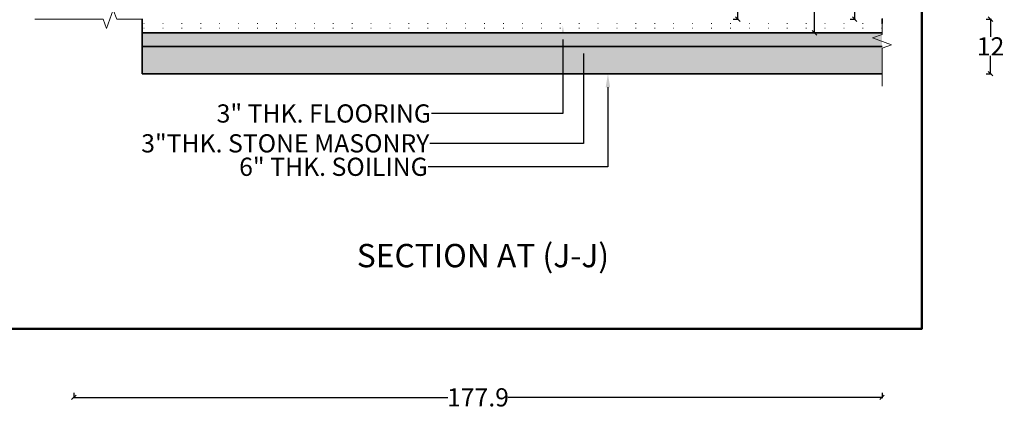
# Model space of a CAD drawing. Units: inches. Extents: x -60 to 284, y -245 to 257.
# Tile 2 of 10: x 55 to 272, y -245 to -159. Entities that reach past the tile are written whole.
import ezdxf
from ezdxf import colors
from ezdxf.entities.mleader import LeaderData, LeaderLine
from ezdxf.math import Vec2, Vec3

# ---------------------------------------------------------------- set-up
doc = ezdxf.new("R2010")
doc.units = ezdxf.units.IN
doc.header["$LTSCALE"] = 0.8
doc.header["$MEASUREMENT"] = 0
doc.linetypes.add('DOT', pattern=[6.35, 0, -6.35])
for name, color, linetype, lineweight in [('A-ANNO-DIMS', 2, 'Continuous', 18), ('A-ANNO-SYMB', 3, 'Continuous', 18), ('A-ANNO-TEXT', 3, 'Continuous', 18), ('A-ANNO-TTLB', 7, 'Continuous', 50), ('A-SECT', 7, 'Continuous', 35), ('A-SECT-OVHD', 8, 'DOT', 18), ('A-SECT-PATT', 8, 'Continuous', 13)]:
    doc.layers.add(name, color=color, linetype=linetype, lineweight=lineweight)
doc.styles.get("Standard").update_dxf_attribs({"font": 'arial.ttf'})
doc.dimstyles.get("Standard").update_dxf_attribs({"dimtxt": 4, "dimasz": 1, "dimexe": 0.18, "dimexo": 0.0625, "dimgap": 0.09, "dimtad": 0, "dimtih": 1, "dimtoh": 1, "dimzin": 0, "dimdsep": 46, "dimlunit": 4, "dimtxsty": 'Standard', "dimblk": 'OBLIQUE', "dimcen": 0.09, "dimadec": 0, "dimazin": 0, "dimtfac": 1, "dimtofl": 0, "dimtmove": 0, "dimatfit": 3, "dimfxl": 1, "dimfxlon": 1, "dimtolj": 1, "dimtzin": 0, "dimarcsym": 0})

# ---------------------------------------------------------------- blocks, each defined once
blk = doc.blocks.new('_Oblique')
at = {"color": 0, "linetype": 'ByBlock', "lineweight": -2}
blk.add_line((-0.5, -0.5), (0.5, 0.5), dxfattribs=at)
blk = doc.blocks.new('*D41')
at = {"layer": 'A-ANNO-DIMS', "color": 0, "lineweight": -2, "ltscale": 0.8, "transparency": 16777216}
for p, q in [((192.1, -91.86), (192.1, -90.68)), ((192.1, -90.86), (193.35, -90.86)), ((202.1, -90.86), (200.85, -90.86)), ((202.1, -91.86), (202.1, -90.68))]:
    blk.add_line(p, q, dxfattribs=at)
at = {"layer": 'Defpoints', "color": 0, "ltscale": 0.8, "transparency": 16777216}
for p in [(192.1, -90.86), (192.1, -168.75), (202.1, -168.75)]:
    blk.add_point(p, dxfattribs=at)
at = {"layer": 'A-ANNO-DIMS', "color": 0, "lineweight": -2, "ltscale": 0.8, "transparency": 16777216, "rotation": 180}
blk.add_blockref('_Oblique', (192.1, -90.86), dxfattribs=at)
at = {"layer": 'A-ANNO-DIMS', "color": 0, "lineweight": -2, "ltscale": 0.8, "transparency": 16777216}
blk.add_blockref('_Oblique', (202.1, -90.86), dxfattribs=at)
at = {"layer": 'A-ANNO-DIMS', "color": 0, "ltscale": 0.8, "transparency": 16777216, "insert": (197.1, -90.86), "char_height": 4, "attachment_point": 5}
blk.add_mtext('\\A1;10"', dxfattribs=at)
blk = doc.blocks.new('*D42')
at = {"layer": 'A-ANNO-DIMS', "color": 0, "lineweight": -2, "ltscale": 0.8, "transparency": 16777216}
for p, q in [((182.1, -91.86), (182.1, -90.68)), ((182.1, -90.86), (183.35, -90.86)), ((192.1, -90.86), (190.85, -90.86)), ((192.1, -91.86), (192.1, -90.68))]:
    blk.add_line(p, q, dxfattribs=at)
at = {"layer": 'Defpoints', "color": 0, "ltscale": 0.8, "transparency": 16777216}
for p in [(182.1, -90.86), (182.1, -162.75), (192.1, -162.75)]:
    blk.add_point(p, dxfattribs=at)
at = {"layer": 'A-ANNO-DIMS', "color": 0, "lineweight": -2, "ltscale": 0.8, "transparency": 16777216, "rotation": 180}
blk.add_blockref('_Oblique', (182.1, -90.86), dxfattribs=at)
at = {"layer": 'A-ANNO-DIMS', "color": 0, "lineweight": -2, "ltscale": 0.8, "transparency": 16777216}
blk.add_blockref('_Oblique', (192.1, -90.86), dxfattribs=at)
at = {"layer": 'A-ANNO-DIMS', "color": 0, "ltscale": 0.8, "transparency": 16777216, "insert": (187.1, -90.86), "char_height": 4, "attachment_point": 5}
blk.add_mtext('\\A1;10"', dxfattribs=at)
blk = doc.blocks.new('*D69')
at = {"layer": 'A-ANNO-DIMS', "color": 0, "lineweight": -2, "ltscale": 0.8, "transparency": 16777216}
for p, q in [((212.15, -46.21), (213.33, -46.21)), ((213.15, -46.21), (213.15, -100.58)), ((213.15, -159.21), (213.15, -104.84)), ((212.15, -159.21), (213.33, -159.21))]:
    blk.add_line(p, q, dxfattribs=at)
at = {"layer": 'Defpoints', "color": 0, "ltscale": 0.8, "transparency": 16777216}
for p in [(212.05, -46.21), (213.15, -46.21), (212.05, -159.21)]:
    blk.add_point(p, dxfattribs=at)
at = {"layer": 'A-ANNO-DIMS', "color": 0, "lineweight": -2, "ltscale": 0.8, "transparency": 16777216}
for p, rotation in [((213.15, -46.21), 90), ((213.15, -159.21), 270)]:
    blk.add_blockref('_Oblique', p, dxfattribs=dict(at, rotation=rotation))
at = {"layer": 'A-ANNO-DIMS', "color": 0, "ltscale": 0.8, "transparency": 16777216, "insert": (213.15, -102.71), "char_height": 4, "attachment_point": 5}
blk.add_mtext('\\A1;9\'-5"', dxfattribs=at)
blk = doc.blocks.new('*D70')
at = {"layer": 'A-ANNO-DIMS', "color": 0, "lineweight": -2, "ltscale": 0.8, "transparency": 16777216}
for p, q in [((229.03, -46.21), (230.21, -46.21)), ((230.03, -46.21), (230.03, -102.08)), ((230.03, -162.21), (230.03, -106.34)), ((229.03, -162.21), (230.21, -162.21))]:
    blk.add_line(p, q, dxfattribs=at)
at = {"layer": 'Defpoints', "color": 0, "ltscale": 0.8, "transparency": 16777216}
for p in [(227.81, -46.21), (230.03, -46.21), (219.24, -162.21)]:
    blk.add_point(p, dxfattribs=at)
at = {"layer": 'A-ANNO-DIMS', "color": 0, "lineweight": -2, "ltscale": 0.8, "transparency": 16777216}
for p, rotation in [((230.03, -46.21), 90), ((230.03, -162.21), 270)]:
    blk.add_blockref('_Oblique', p, dxfattribs=dict(at, rotation=rotation))
at = {"layer": 'A-ANNO-DIMS', "color": 0, "ltscale": 0.8, "transparency": 16777216, "insert": (230.03, -104.21), "char_height": 4, "attachment_point": 5}
blk.add_mtext('\\A1;9\'-8"', dxfattribs=at)
blk = doc.blocks.new('*D71')
at = {"layer": 'A-ANNO-DIMS', "color": 0, "lineweight": -2, "ltscale": 0.8, "transparency": 16777216}
for p, q in [((237.88, -38.61), (239.06, -38.61)), ((238.88, -38.61), (238.88, -94.1)), ((238.88, -159.21), (238.88, -103.72)), ((237.88, -159.21), (239.06, -159.21))]:
    blk.add_line(p, q, dxfattribs=at)
at = {"layer": 'Defpoints', "color": 0, "ltscale": 0.8, "transparency": 16777216}
for p in [(235.46, -38.61), (238.88, -38.61), (235.46, -159.21)]:
    blk.add_point(p, dxfattribs=at)
at = {"layer": 'A-ANNO-DIMS', "color": 0, "lineweight": -2, "ltscale": 0.8, "transparency": 16777216}
for p, rotation in [((238.88, -38.61), 90), ((238.88, -159.21), 270)]:
    blk.add_blockref('_Oblique', p, dxfattribs=dict(at, rotation=rotation))
at = {"layer": 'A-ANNO-DIMS', "color": 0, "ltscale": 0.8, "transparency": 16777216, "insert": (238.88, -98.91), "char_height": 4, "attachment_point": 5}
blk.add_mtext('\\A1;10\'-0{\\H1x;\\S1/2;}"', dxfattribs=at)
blk = doc.blocks.new('*D105')
at = {"layer": 'A-ANNO-DIMS', "color": 0, "lineweight": -2, "ltscale": 0.8, "transparency": 16777216}
for p, q in [((67.01, -241.38), (67.01, -242.56)), ((67.01, -242.38), (149.3, -242.38)), ((244.9, -242.38), (162.61, -242.38)), ((244.9, -241.38), (244.9, -242.56))]:
    blk.add_line(p, q, dxfattribs=at)
at = {"layer": 'Defpoints', "color": 0, "ltscale": 0.8, "transparency": 16777216}
for p in [(67.01, -159.21), (244.9, -171.21), (244.9, -242.38)]:
    blk.add_point(p, dxfattribs=at)
at = {"layer": 'A-ANNO-DIMS', "color": 0, "lineweight": -2, "ltscale": 0.8, "transparency": 16777216, "rotation": 180}
blk.add_blockref('_Oblique', (67.01, -242.38), dxfattribs=at)
at = {"layer": 'A-ANNO-DIMS', "color": 0, "lineweight": -2, "ltscale": 0.8, "transparency": 16777216}
blk.add_blockref('_Oblique', (244.9, -242.38), dxfattribs=at)
at = {"layer": 'A-ANNO-DIMS', "color": 0, "ltscale": 0.8, "transparency": 16777216, "insert": (155.96, -242.38), "char_height": 4, "attachment_point": 5}
blk.add_mtext('\\A1;177.9', dxfattribs=at)
blk = doc.blocks.new('*D108')
at = {"layer": 'A-ANNO-DIMS', "color": 0, "lineweight": -2, "ltscale": 0.8, "transparency": 16777216}
for p, q in [((267.79, -159.21), (268.97, -159.21)), ((268.79, -159.21), (268.79, -163.11)), ((268.79, -171.21), (268.79, -167.31)), ((267.79, -171.21), (268.97, -171.21))]:
    blk.add_line(p, q, dxfattribs=at)
at = {"layer": 'Defpoints', "color": 0, "ltscale": 0.8, "transparency": 16777216}
for p in [(244.9, -159.21), (244.9, -171.21), (268.79, -171.21)]:
    blk.add_point(p, dxfattribs=at)
at = {"layer": 'A-ANNO-DIMS', "color": 0, "lineweight": -2, "ltscale": 0.8, "transparency": 16777216}
for p, rotation in [((268.79, -159.21), 90), ((268.79, -171.21), 270)]:
    blk.add_blockref('_Oblique', p, dxfattribs=dict(at, rotation=rotation))
at = {"layer": 'A-ANNO-DIMS', "color": 0, "ltscale": 0.8, "transparency": 16777216, "insert": (268.79, -165.21), "char_height": 4, "attachment_point": 5}
blk.add_mtext('\\A1;12', dxfattribs=at)

msp = doc.modelspace()

# ---------------------------------------------------------------- hatches: boundary and pattern name
at = {"layer": 'A-SECT-PATT', "ltscale": 0.8}
h = msp.add_hatch(dxfattribs=at)
h.set_pattern_fill('AR-CONC', color=256, scale=0.8)
h.set_pattern_definition([(50, (0, 145.9847), (5.73808, -0.502017), [0.6, -6.6]), (355, (0, 145.985), (-1.11001, 6.01754), [0.48, -5.28]), (100.4514, (0.478, 145.943), (4.62807, 5.51552), [0.50992, -5.60914]), (46.1842, (0, 147.585), (8.53793, -1.32415), [0.9, -9.9]), (96.6356, (0.7115, 147.474), (7.4773, 7.79295), [0.76488, -8.41371]), (351.1842, (0, 147.585), (7.4773, 7.79295), [0.72, -7.92]), (21, (0.8, 147.1847), (4.775256, -3.22095), [0.6, -6.6]), (326, (0.8, 147.185), (1.94652, 5.8012), [0.48, -5.28]), (71.4514, (1.198, 146.9163), (6.72178, 2.58025), [0.50992, -5.60914]), (37.5, (0, 145.9847), (0.097279, 2.663151), [0, -5.216, 0, -5.36, 0, -5.3]), (7.5, (0, 145.9847), (2.104556, 3.155294), [0, -3.056, 0, -5.096, 0, -2.02]), (327.5, (-1.784, 145.9847), (4.27058, -0.180439), [0, -2, 0, -6.24, 0, -8.28]), (317.5, (-2.584, 145.9847), (4.66549, 0.80084), [0, -2.6, 0, -4.144, 0, -5.88])])
h.paths.add_polyline_path([(244.8977, -162.2089), (82.0139, -162.2089), (82.0139, -165.2089), (244.8977, -165.2089)])
h = msp.add_hatch(dxfattribs=at)
h.set_pattern_fill('GRAVEL', color=256, scale=6)
h.set_pattern_definition([(228.01279, (4.32, 151.9847), (-48, -54), [0.807216, -79.91453]), (184.96974, (3.78, 151.38472), (72, 6), [1.38521, -137.13555]), (132.51045, (2.4, 151.2647), (60, -66), [0.97673, -96.696196]), (267.27369, (0.06, 149.76472), (6, 120), [1.26143, -124.88135]), (292.833654, (0, 148.50472), (-30, 72), [1.23693, -122.45624]), (357.27369, (0.48, 147.36472), (-120, 6), [1.26143, -124.88135]), (37.69424, (1.74, 147.30472), (-78, -60), [1.668174, -165.14909]), (72.25533, (3.06, 148.32472), (42, 132), [1.57493, -155.91793]), (121.429566, (3.54, 149.82472), (-48, 78), [1.2657, -125.30444]), (175.23636, (2.88, 150.9047), (66, -6), [1.44499, -70.804575]), (222.39744, (1.44, 151.02472), (-72, -66), [1.86869, -185.00025]), (138.81407, (6, 149.7047), (-42, 36), [0.637806, -63.14307]), (171.469234, (5.52, 150.12472), (78, -12), [1.21342, -120.12907]), (225, (4.32, 150.3047), (-7e-16, -6), [0.84853, -7.636755]), (203.1986, (3.9, 151.0247), (30, 12), [0.45695, -45.23769]), (291.8014, (3.48, 150.8447), (-6, 18), [0.64622, -31.66477]), (30.96376, (3.72, 150.2447), (18, 12), [1.04957, -33.93614]), (161.56505, (4.62, 150.7847), (12, -6), [0.75895, -18.21472]), (16.38954, (0, 150.8447), (60, 18), [1.0632, -105.25707]), (70.34618, (1.02, 151.1447), (-24, -66), [0.891966, -88.30445]), (293.1986, (4.62, 151.9847), (-12, 30), [0.91389, -44.78075]), (343.61046, (4.98, 151.1447), (-60, 18), [1.0632, -105.25707]), (339.44395, (0, 147.1247), (-30, 12), [1.02528, -50.23874]), (294.77514, (0.96, 146.7647), (-30, 66), [0.85907, -85.04786]), (66.8014, (4.68, 145.9847), (12, 30), [0.91389, -44.78075]), (17.35402, (5.04, 146.8247), (-78, -24), [1.005786, -99.57254]), (69.44395, (1.74, 145.9847), (-12, -30), [0.51264, -50.75138]), (101.30993, (4.32, 145.9847), (-6, 24), [0.30594, -30.28818]), (165.96376, (4.26, 146.2847), (18, -6), [1.23693, -23.5017]), (186.00901, (3.06, 146.58472), (60, 6), [1.1463, -113.48354]), (303.69007, (3.72, 149.7047), (-6, 12), [0.86533, -20.767976]), (353.157227, (4.2, 148.98472), (102, -12), [1.510764, -149.565376]), (60.9454, (5.7, 148.8047), (-24, -42), [0.617736, -61.156045]), (90, (6, 149.345), (-6, 6), [0.36, -5.64]), (120.25644, (2.94, 146.7647), (24, -42), [0.833544, -82.52112]), (48.01279, (2.52, 147.4847), (48, 54), [1.61443, -79.10731]), (0, (3.6, 148.685), (6, 6), [1.56, -4.44]), (325.30485, (5.16, 148.6847), (60, -42), [0.948684, -93.919646]), (254.0546, (5.94, 148.1447), (-6, -24), [0.87361, -42.80705]), (207.645975, (5.7, 147.30472), (-114, -60), [1.42239, -140.816845]), (175.42608, (4.44, 146.64472), (-78, 6), [1.504794, -148.97444])])
h.paths.add_polyline_path([(244.8977, -165.2089), (82.0139, -165.2089), (82.0139, -171.2089), (244.8977, -171.2089)])

# ---------------------------------------------------------------- linework, layer by layer
at = {"layer": 'A-ANNO-SYMB', "ltscale": 0.8}
for points in [[(82.1939, -159.2089), (76.4394, -159.2089), (75.6894, -157.1482), (74.1894, -161.2695), (73.4394, -159.2089), (58.3996, -159.2089)], [(244.8977, -159.0289), (244.8977, -162.6103), (242.8371, -163.3603), (246.9583, -164.8603), (244.8977, -165.6103), (244.8977, -173.978)]]:
    msp.add_lwpolyline(points, dxfattribs=at)
at = {"layer": 'A-ANNO-TTLB', "ltscale": 0.8}
msp.add_lwpolyline([(-36.7489, -7.223), (253.6882, -7.223), (253.6882, -227.2835), (-36.7489, -227.2835)], close=True, dxfattribs=at)
at = {"layer": 'A-SECT', "ltscale": 0.8}
for p, q in [((82.0139, -159.2089), (82.0139, -171.2089)), ((244.8977, -159.2089), (244.8977, -160.2089)), ((244.8977, -162.2089), (82.0139, -162.2089)), ((244.8977, -165.2089), (82.0139, -165.2089)), ((244.8977, -171.2089), (82.0139, -171.2089))]:
    msp.add_line(p, q, dxfattribs=at)
at = {"layer": 'A-SECT-OVHD', "ltscale": 0.8}
for p, q in [((244.8977, -160.2089), (82.0139, -160.2089)), ((244.8977, -161.2089), (82.0139, -161.2089))]:
    msp.add_line(p, q, dxfattribs=at)

# ---------------------------------------------------------------- texts
at = {"layer": 'A-ANNO-TEXT', "ltscale": 0.8, "insert": (129.2829, -208.6458), "char_height": 5.134626, "attachment_point": 1}
msp.add_mtext_dynamic_manual_height_columns('{SECTION AT (J-J)}', width=125.222392, gutter_width=1.2837, heights=[0], dxfattribs=at)

# ---------------------------------------------------------------- dimensions: what is measured, and where the dimension line sits
at = {"layer": 'A-ANNO-DIMS', "ltscale": 0.8}
for base, p1, p2, override, picture, middle in [((238.8784, -38.6089), (235.4628, -159.2089), (235.4628, -38.6089), {"dimclrd": 0, "dimclre": 0, "dimclrt": 0}, '*D71', (238.8784, -98.9089)), ((213.1492, -46.2089), (212.0462, -159.2089), (212.0462, -46.2089), {"dimclrd": 0, "dimclre": 0, "dimclrt": 0}, '*D69', (213.1492, -102.7089)), ((230.0275, -46.2089), (219.2361, -162.2089), (227.8081, -46.2089), {"dimclrd": 0, "dimclre": 0, "dimclrt": 0}, '*D70', (230.0275, -104.2089)), ((268.7882, -171.2089), (244.8977, -159.2089), (244.8977, -171.2089), {"dimdec": 0, "dimlfac": 1, "dimrnd": 0, "dimzin": 0, "dimdsep": 46, "dimlunit": 2}, '*D108', (268.7882, -165.2089))]:
    dim = msp.add_linear_dim(base=base, p1=p1, p2=p2, angle=90, dimstyle='Standard', override=override, dxfattribs=at)
    dim.commit()
    dim.dimension.update_dxf_attribs({"geometry": picture, "text_midpoint": middle})
for base, p1, p2, override, picture, middle in [((182.1002, -90.8616), (192.1002, -162.7549), (182.1002, -162.7549), {"dimclrd": 0, "dimclre": 0, "dimclrt": 0}, '*D42', (187.1002, -90.8616)), ((192.1002, -90.8616), (202.1002, -168.7549), (192.1002, -168.7549), {"dimclrd": 0, "dimclre": 0, "dimclrt": 0}, '*D41', (197.1002, -90.8616)), ((244.8977, -242.3835), (67.0139, -159.2089), (244.8977, -171.2089), {"dimdec": 1, "dimlfac": 1, "dimrnd": 0, "dimzin": 0, "dimdsep": 46, "dimlunit": 2}, '*D105', (155.9558, -242.3835))]:
    dim = msp.add_linear_dim(base=base, p1=p1, p2=p2, dimstyle='Standard', override=override, dxfattribs=at)
    dim.commit()
    dim.dimension.update_dxf_attribs({"geometry": picture, "text_midpoint": middle})

# ---------------------------------------------------------------- leaders
at = {"layer": 'A-ANNO-TEXT', "ltscale": 0.8}
ml = msp.add_multileader_mtext('Standard', dxfattribs=at)
ml.set_content('15" THK. STONE MASONRY', color=256)
ml.set_leader_properties()
ml.build(insert=Vec2(0, 0))
ml.multileader.update_dxf_attribs({"dogleg_length": 0.36, "arrow_head_size": 3})
ctx = ml.context
ctx.base_point, ctx.arrow_head_size, ctx.landing_gap_size, ctx.plane_origin = Vec3(93.0628, -148.337), 3, 0.09, Vec3(81.8179, -148.337)
notes = []
notes.append((ctx, [(0, (1, 1, 0), (92.7028, -148.337), (1, 0), 0.36, [(0, [(81.8179, -148.337)], 0, [])])]))
ctx.mtext.insert, ctx.mtext.flow_direction = Vec3(93.1528, -146.3029), 5
ml = msp.add_multileader_mtext('Standard', dxfattribs=at)
ml.set_content('3" THK. FLOORING', color=256)
ml.set_leader_properties()
ml.build(insert=Vec2(0, 0))
ml.multileader.update_dxf_attribs({"dogleg_length": 0.36, "arrow_head_size": 3})
ctx = ml.context
ctx.base_point, ctx.arrow_head_size, ctx.landing_gap_size, ctx.plane_origin = Vec3(96.0004, -179.9957), 3, 0.09, Vec3(174.6475, -160.6891)
ctx.text_align_type = 2
notes.append((ctx, [(0, (1, 1, 0), (146.0656, -179.9957), (-1, 0), 0.36, [(0, [(174.6475, -160.6891), (174.6475, -179.9957)], 0, [])])]))
ctx.mtext.insert, ctx.mtext.alignment, ctx.mtext.flow_direction = Vec3(145.6156, -177.9603), 3, 5
ml = msp.add_multileader_mtext('Standard', dxfattribs=at)
ml.set_content('3"THK. STONE MASONRY', color=256)
ml.set_leader_properties()
ml.build(insert=Vec2(0, 0))
ml.multileader.update_dxf_attribs({"dogleg_length": 0.36, "arrow_head_size": 3})
ctx = ml.context
ctx.base_point, ctx.arrow_head_size, ctx.landing_gap_size, ctx.plane_origin = Vec3(77.0155, -186.5647), 3, 0.09, Vec3(179.1706, -163.7541)
ctx.text_align_type = 2
notes.append((ctx, [(0, (1, 1, 0), (145.7056, -186.5647), (-1, 0), 0.36, [(0, [(179.1706, -163.7541), (179.1706, -186.5647)], 0, [])])]))
ctx.mtext.insert, ctx.mtext.alignment, ctx.mtext.flow_direction = Vec3(145.2556, -184.5292), 3, 5
ml = msp.add_multileader_mtext('Standard', dxfattribs=at)
ml.set_content('6" THK. SOILING', color=256)
ml.set_leader_properties()
ml.build(insert=Vec2(0, 0))
ml.multileader.update_dxf_attribs({"dogleg_length": 0.36, "arrow_head_size": 3})
ctx = ml.context
ctx.base_point, ctx.arrow_head_size, ctx.landing_gap_size, ctx.plane_origin = Vec3(101.7715, -191.7174), 3, 0.09, Vec3(184.5639, -171.2089)
ctx.text_align_type = 2
notes.append((ctx, [(0, (1, 1, 0), (145.3456, -191.7174), (-1, 0), 0.36, [(0, [(184.5639, -171.2089), (184.5639, -191.7174)], 0, [])])]))
ctx.mtext.insert, ctx.mtext.alignment, ctx.mtext.flow_direction = Vec3(144.8956, -189.6833), 3, 5
for ctx, leaders in notes:
    for number, flags, end, landing, length, lines in leaders:
        leader = LeaderData()
        leader.index, (leader.has_last_leader_line, leader.has_dogleg_vector, leader.attachment_direction) = number, flags
        leader.last_leader_point, leader.dogleg_vector, leader.dogleg_length = Vec3(end), Vec3(landing), length
        for number, points, colour, breaks in lines:
            line = LeaderLine()
            line.index, line.vertices, line.color, line.breaks = number, Vec3.list(points), colors.encode_raw_color(colour), breaks
            leader.lines.append(line)
        ctx.leaders.append(leader)

doc.saveas('drawing.dxf')
